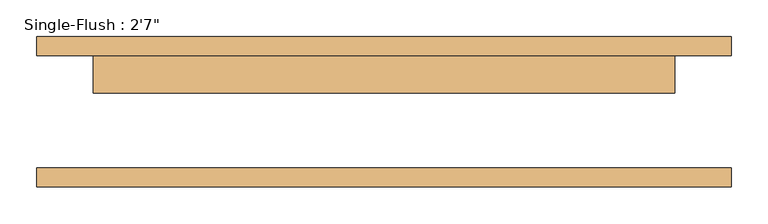
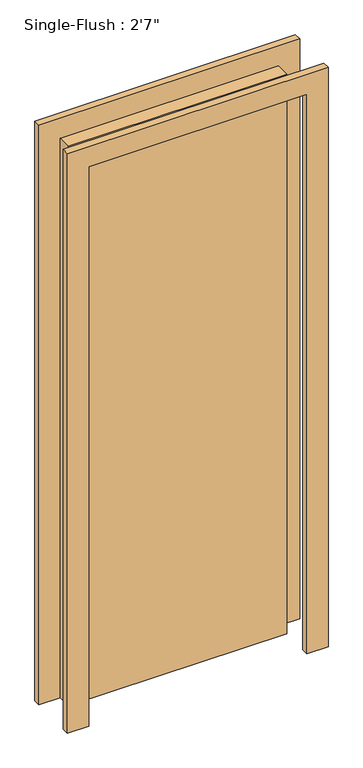
"""IFC4 building model written with IfcOpenShell, lengths in millimetres: door geometry."""

from ifc_helpers import new_model, si_unit, frame, origin, origin_with_axes, place, context, project, spatial, polyline, outline, extrude, source, transform, mapped, element, save


def door_b804d09e(model_context):
    return source(origin(), model_context, "Body", "SweptSolid", [
        extrude(outline(polyline([(2209.8, -469.9), (0.0, -469.9), (0.0, -393.7), (2133.6, -393.7), (2133.6, 393.7), (0.0, 393.7), (0.0, 469.9), (2209.8, 469.9), (2209.8, -469.9)])), frame((0.0, 76.2, 0.0), z_axis=(0.0, 1.0, 0.0), x_axis=(0.0, 0.0, 1.0)), (0.0, 0.0, 1.0), 25.4),
        extrude(outline(polyline([(2209.8, 469.9), (2209.8, -469.9), (0.0, -469.9), (0.0, -393.7), (2133.6, -393.7), (2133.6, 393.7), (0.0, 393.7), (0.0, 469.9), (2209.8, 469.9)])), frame((0.0, -101.6, 0.0), z_axis=(0.0, 1.0, 0.0), x_axis=(0.0, 0.0, 1.0)), (0.0, 0.0, 1.0), 25.4),
        extrude(outline(polyline([(393.7, 25.4), (-393.7, 25.4), (-393.7, 76.2), (393.7, 76.2), (393.7, 25.4)])), origin_with_axes(), (0.0, 0.0, 1.0), 2133.6),
    ])


if __name__ == "__main__":
    model = new_model("IFC4")
    model_context = context("Model", 3, world=origin())
    ifc_project = project(units=[si_unit("LENGTHUNIT", "METRE", prefix="MILLI")], contexts=[model_context])
    site = spatial("IfcSite", under=ifc_project)
    building = spatial("IfcBuilding", under=site)
    placement = place(None, origin())
    door_shape = door_b804d09e(model_context)
    element("IfcDoor", 1, ObjectType="Single-Flush : 2'7\"", at=placement, inside=building, context=model_context, shape_type="MappedRepresentation", body=[
        mapped(door_shape, transform((0.0, 0.0, 0.0), x_axis=(1.0, 0.0, 0.0), y_axis=(0.0, 1.0, 0.0), z_axis=(0.0, 0.0, 1.0))),
    ])
    save(model, "model.ifc")

# Revit data of these elements
# Type "Single-Flush : 2'7\""
#   Type Mark = "8"
#   Construction Type Id = "MDOOR"
#   Assembly Code = "C1020"
#   Analytic Construction = "Metal"
#   Thickness = 0' - 2"
#   Heat Transfer Coefficient (U) = 0.651978 BTU/(h·ft²·°F)
#   Height = 7' - 0"
#   Trim Projection Ext = 0' - 1"
#   Trim Projection Int = 0' - 1"
#   Trim Width = 0' - 3"
#   Width = 2' - 7"
#   Define Thermal Properties by = 1
#   Door Material = Door - Panel
#   Frame Material = Door - Frame
#   Visual Light Transmittance = 0
#   Solar Heat Gain Coefficient = 0
#   Function = (empty or 0)
#   Wall Closure = (empty or 0)
# Element 1 (IfcDoor, "Single-Flush : 2'7\"")
#   Materials on its faces: "Door - Frame", "Door - Panel"
# Materials
#   "Door - Panel": class "Wood", colour RGB 210 159 95, transparency 0, Cost = 0
#   "Door - Frame": colour RGB 118 70 51, transparency 0, Cost = 0
